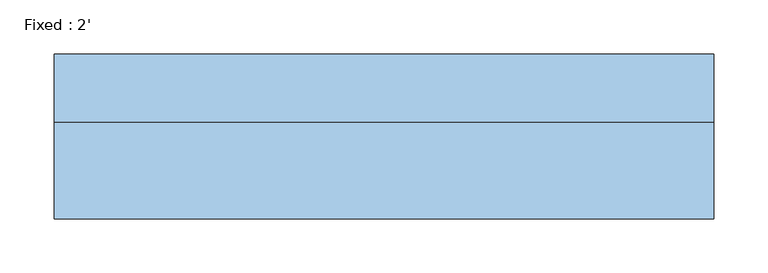
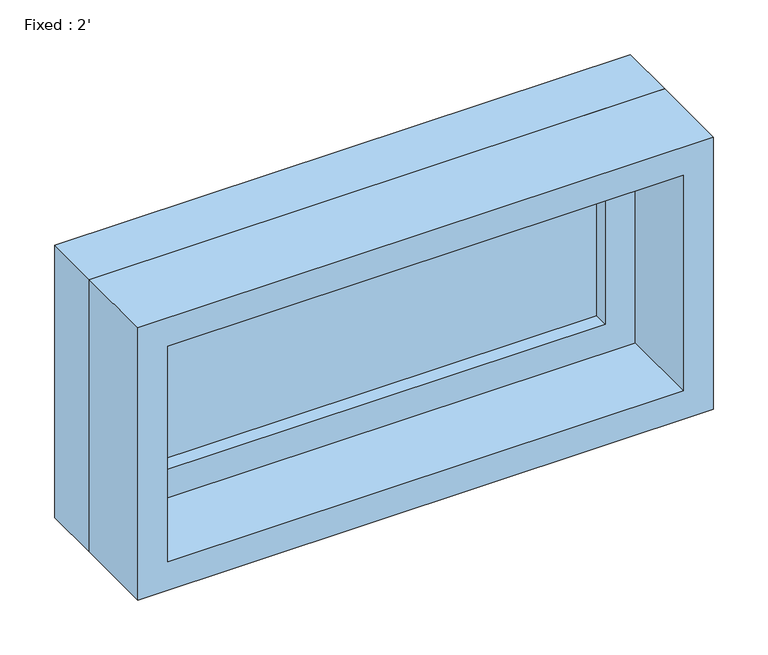
"""IFC4 building model written with IfcOpenShell, lengths in millimetres: window geometry, Fixed : 2'."""

from ifc_helpers import new_model, si_unit, frame, origin, place, context, project, spatial, polyline, outline, extrude, source, transform, mapped, element, save


def fixed_2_65c13adb(model_context):
    return source(origin(), model_context, "Body", "SweptSolid", [
        extrude(outline(polyline([(203.2, 28.575), (-279.4, 28.575), (-279.4, 41.275), (203.2, 41.275), (203.2, 28.575)])), frame((0.0, 0.0, 977.9), z_axis=(0.0, 0.0, 1.0), x_axis=(1.0, 0.0, 0.0)), (0.0, 0.0, 1.0), 177.8),
        extrude(outline(polyline([(1200.15, -323.85), (933.45, -323.85), (933.45, 247.65), (1200.15, 247.65), (1200.15, -323.85)]), holes=[polyline([(1155.7, -279.4), (1155.7, 203.2), (977.9, 203.2), (977.9, -279.4), (1155.7, -279.4)])]), frame((0.0, 12.7, 0.0), z_axis=(0.0, 1.0, 0.0), x_axis=(0.0, 0.0, 1.0)), (0.0, 0.0, 1.0), 44.45),
        extrude(outline(polyline([(1219.2, -342.9), (914.4, -342.9), (914.4, 266.7), (1219.2, 266.7), (1219.2, -342.9)]), holes=[polyline([(1187.45, -311.15), (1187.45, 234.95), (946.15, 234.95), (946.15, -311.15), (1187.45, -311.15)])]), frame((0.0, -76.2, 0.0), z_axis=(0.0, 1.0, 0.0), x_axis=(0.0, 0.0, 1.0)), (0.0, 0.0, 1.0), 88.9),
        extrude(outline(polyline([(1219.2, 266.7), (1219.2, -342.9), (914.4, -342.9), (914.4, 266.7), (1219.2, 266.7)]), holes=[polyline([(1200.15, 247.65), (933.45, 247.65), (933.45, -323.85), (1200.15, -323.85), (1200.15, 247.65)])]), frame((0.0, 12.7, 0.0), z_axis=(0.0, 1.0, 0.0), x_axis=(0.0, 0.0, 1.0)), (0.0, 0.0, 1.0), 63.5),
    ])


if __name__ == "__main__":
    model = new_model("IFC4")
    model_context = context("Model", 3, world=origin())
    ifc_project = project(units=[si_unit("LENGTHUNIT", "METRE", prefix="MILLI")], contexts=[model_context])
    site = spatial("IfcSite", under=ifc_project)
    building = spatial("IfcBuilding", under=site)
    placement = place(None, origin())
    fixed_2_shape = fixed_2_65c13adb(model_context)
    element("IfcWindow", 1, ObjectType="Fixed : 2'", at=placement, inside=building, context=model_context, shape_type="MappedRepresentation", body=[
        mapped(fixed_2_shape, transform((0.0, 0.0, 0.0), x_axis=(1.0, 0.0, 0.0), y_axis=(0.0, 1.0, 0.0), z_axis=(0.0, 0.0, 1.0))),
    ])
    save(model, "model.ifc")

# Revit data of these elements
# Type "Fixed : 2'"
#   Type Mark = "16"
#   Assembly Code = "B2020100"
#   Height = 1' - 0"
#   Default Sill Height = 3' - 0"
#   Width = 2' - 0"
#   Window Inset = 0' - 0 3/4"
#   Glass Pane Material = Glass
#   Sash Material = Sash
#   Wall Closure = (empty or 0)
# Element 1 (IfcWindow, "Fixed : 2'")
#   Materials on its faces: "Sash", "Glass"
# Materials
#   "Glass": class "Glass", colour RGB 218 227 224, transparency 0.85, Description = "Soda Lime Glass", Cost = 0
#   "Sash": class "Wood", colour RGB 136 99 55, transparency 0
